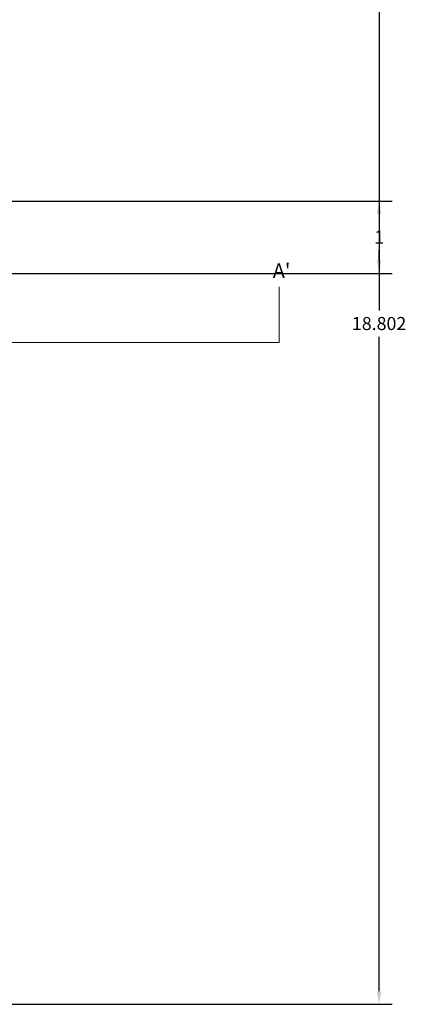
# Model space of a CAD drawing. Units: metres. Extents: x 2031 to 2061.8, y 1886.4 to 1909.8.
# Tile 9 of 10: x 2056.5 to 2061.8, y 1888.3 to 1901.9. Entities that reach past the tile are written whole.
import ezdxf

# ---------------------------------------------------------------- set-up
doc = ezdxf.new("R2010")
doc.units = ezdxf.units.M
doc.layers.add('A-ANNO-DIMS', color=2, linetype='Continuous', lineweight=18)
doc.layers.add('A-ANNO-SYMB', color=7, linetype='Continuous', lineweight=18)
doc.styles.get("Standard").update_dxf_attribs({"font": 'arial.ttf'})
doc.dimstyles.get("Standard").update_dxf_attribs({"dimtxt": 0.18, "dimasz": 0.18, "dimexe": 0.18, "dimexo": 0.0625, "dimgap": 0.09, "dimtad": 0, "dimtih": 1, "dimtoh": 1, "dimdec": 4, "dimzin": 0, "dimdsep": 46, "dimtxsty": 'Standard', "dimcen": 0.09, "dimadec": 0, "dimazin": 0, "dimtfac": 1, "dimtdec": 4, "dimtofl": 0, "dimtmove": 0, "dimatfit": 3, "dimfxl": 1, "dimtolj": 1, "dimtzin": 0, "dimarcsym": 0})

# ---------------------------------------------------------------- blocks, each defined once
blk = doc.blocks.new('*D45')
at = {"layer": 'A-ANNO-DIMS', "color": 0, "lineweight": -2, "transparency": 16777216}
for p, q in [((2047.556, 1907.081), (2061.614, 1907.081)), ((2061.434, 1906.901), (2061.434, 1897.862)), ((2061.434, 1888.459), (2061.434, 1897.498)), ((2054.286, 1888.279), (2061.614, 1888.279))]:
    blk.add_line(p, q, dxfattribs=at)
at = {"layer": 'A-ANNO-DIMS', "color": 0, "transparency": 16777216}
for points in [[(2061.404, 1906.901), (2061.464, 1906.901), (2061.434, 1907.081)], [(2061.404, 1888.459), (2061.464, 1888.459), (2061.434, 1888.279)]]:
    blk.add_solid(points, dxfattribs=at)
at = {"layer": 'Defpoints', "color": 0, "transparency": 16777216}
for p in [(2047.494, 1907.081), (2061.434, 1907.081), (2054.224, 1888.279)]:
    blk.add_point(p, dxfattribs=at)
at = {"layer": 'A-ANNO-DIMS', "color": 0, "transparency": 16777216, "insert": (2061.434, 1897.68), "char_height": 0.18, "attachment_point": 5}
blk.add_mtext('\\A1;18.802', dxfattribs=at)
blk = doc.blocks.new('*D57')
at = {"layer": 'A-ANNO-DIMS', "color": 0, "lineweight": -2, "transparency": 16777216}
for p, q in [((2040.478, 1899.371), (2061.614, 1899.371)), ((2061.434, 1899.191), (2061.434, 1899.052)), ((2061.434, 1898.551), (2061.434, 1898.691)), ((2040.478, 1898.371), (2061.614, 1898.371))]:
    blk.add_line(p, q, dxfattribs=at)
at = {"layer": 'A-ANNO-DIMS', "color": 0, "transparency": 16777216}
for points in [[(2061.404, 1899.191), (2061.464, 1899.191), (2061.434, 1899.371)], [(2061.404, 1898.551), (2061.464, 1898.551), (2061.434, 1898.371)]]:
    blk.add_solid(points, dxfattribs=at)
at = {"layer": 'Defpoints', "color": 0, "transparency": 16777216}
for p in [(2040.416, 1899.371), (2061.434, 1899.371), (2040.416, 1898.371)]:
    blk.add_point(p, dxfattribs=at)
at = {"layer": 'A-ANNO-DIMS', "color": 0, "transparency": 16777216, "insert": (2061.434, 1898.871), "char_height": 0.18, "attachment_point": 5}
blk.add_mtext('\\A1;1', dxfattribs=at)

msp = doc.modelspace()

# ---------------------------------------------------------------- linework, layer by layer
at = {"layer": 'A-ANNO-SYMB'}
for p, q in [((2060.0534, 1897.42), (2060.0534, 1898.1861)), ((2033.1258, 1897.42), (2060.0534, 1897.42))]:
    msp.add_line(p, q, dxfattribs=at)

# ---------------------------------------------------------------- texts
at = {"layer": 'A-ANNO-SYMB', "insert": (2059.9679, 1898.3104), "char_height": 0.2, "attachment_point": 7}
msp.add_mtext_dynamic_manual_height_columns("A'", width=2.30233, gutter_width=12.5, heights=[0], dxfattribs=at)

# ---------------------------------------------------------------- dimensions: what is measured, and where the dimension line sits
at = {"layer": 'A-ANNO-DIMS'}
for base, p1, p2, override, picture, middle in [((2061.4344, 1907.0812), (2054.2239, 1888.2791), (2047.4939, 1907.0812), {"dimdec": 3, "dimlfac": 1, "dimrnd": 0, "dimzin": 0, "dimdsep": 46, "dimlunit": 2}, '*D45', (2061.4344, 1897.6801)), ((2061.4344, 1899.3712), (2040.4157, 1898.3712), (2040.4157, 1899.3712), {"dimdec": 0, "dimlfac": 1, "dimrnd": 0, "dimzin": 0, "dimdsep": 46, "dimlunit": 2}, '*D57', (2061.4344, 1898.8712))]:
    dim = msp.add_linear_dim(base=base, p1=p1, p2=p2, angle=90, dimstyle='Standard', override=override, dxfattribs=at)
    dim.commit()
    dim.dimension.update_dxf_attribs({"geometry": picture, "text_midpoint": middle})

doc.saveas('drawing.dxf')
